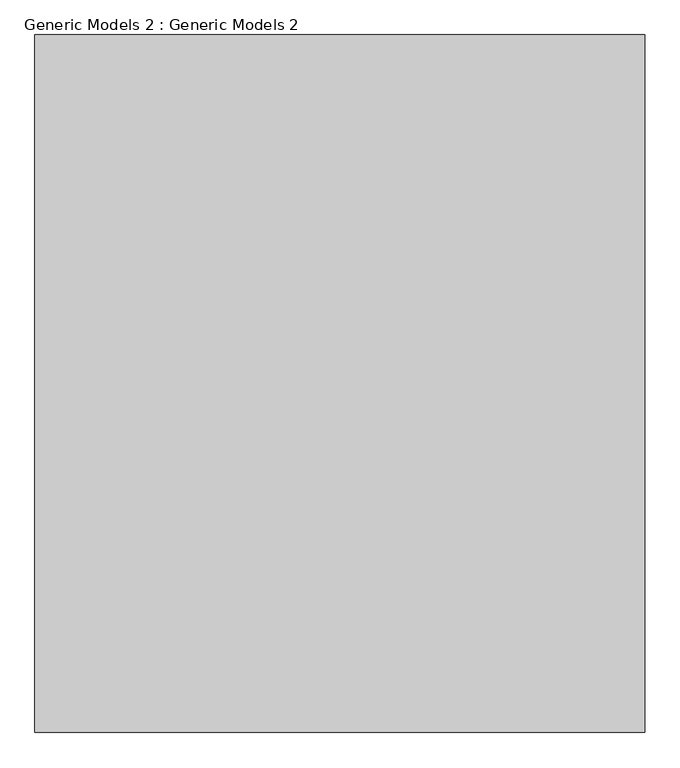
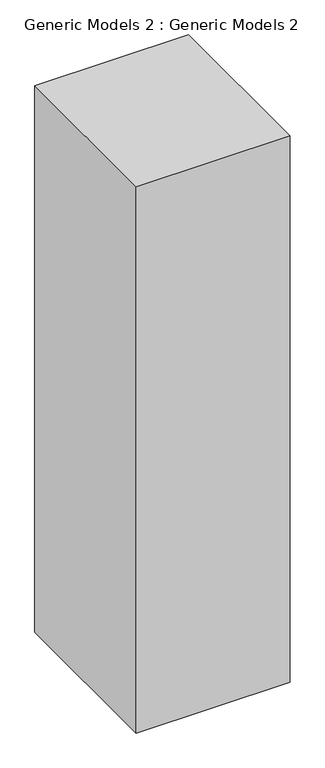
"""IFC4 building model written with IfcOpenShell, lengths in millimetres: proxy geometry, Generic Models 2 : Generic Models 2."""

from ifc_helpers import new_model, si_unit, frame, origin, place, context, project, spatial, polyline, outline, extrude, source, transform, mapped, element, save


def generic_models_2_generic_models_2_1c1dda24(model_context):
    return source(origin(), model_context, "Body", "SweptSolid", [
        extrude(outline(polyline([(4163.3104739, -8641.1821053), (4163.3104739, -9760.0213812), (3185.4072133, -9760.0213812), (3185.4072133, -8641.1821053), (4163.3104739, -8641.1821053)])), frame((0.0, 0.0, 3784.9309605), z_axis=(0.0, 0.0, 1.0), x_axis=(1.0, 0.0, 0.0)), (0.0, 0.0, 1.0), 3676.0971887),
    ])


if __name__ == "__main__":
    model = new_model("IFC4")
    model_context = context("Model", 3, world=origin())
    ifc_project = project(units=[si_unit("LENGTHUNIT", "METRE", prefix="MILLI")], contexts=[model_context])
    site = spatial("IfcSite", under=ifc_project)
    building = spatial("IfcBuilding", under=site)
    placement = place(None, origin())
    generic_models_2_generic_models_2_shape = generic_models_2_generic_models_2_1c1dda24(model_context)
    element("IfcBuildingElementProxy", 1, Name="Generic Models 2 : Generic Models 2", ObjectType="Generic Models 2 : Generic Models 2", at=placement, inside=building, context=model_context, shape_type="MappedRepresentation", body=[
        mapped(generic_models_2_generic_models_2_shape, transform((0.0, 0.0, 0.0), x_axis=(1.0, 0.0, 0.0), y_axis=(0.0, 1.0, 0.0), z_axis=(0.0, 0.0, 1.0))),
    ])
    save(model, "model.ifc")
